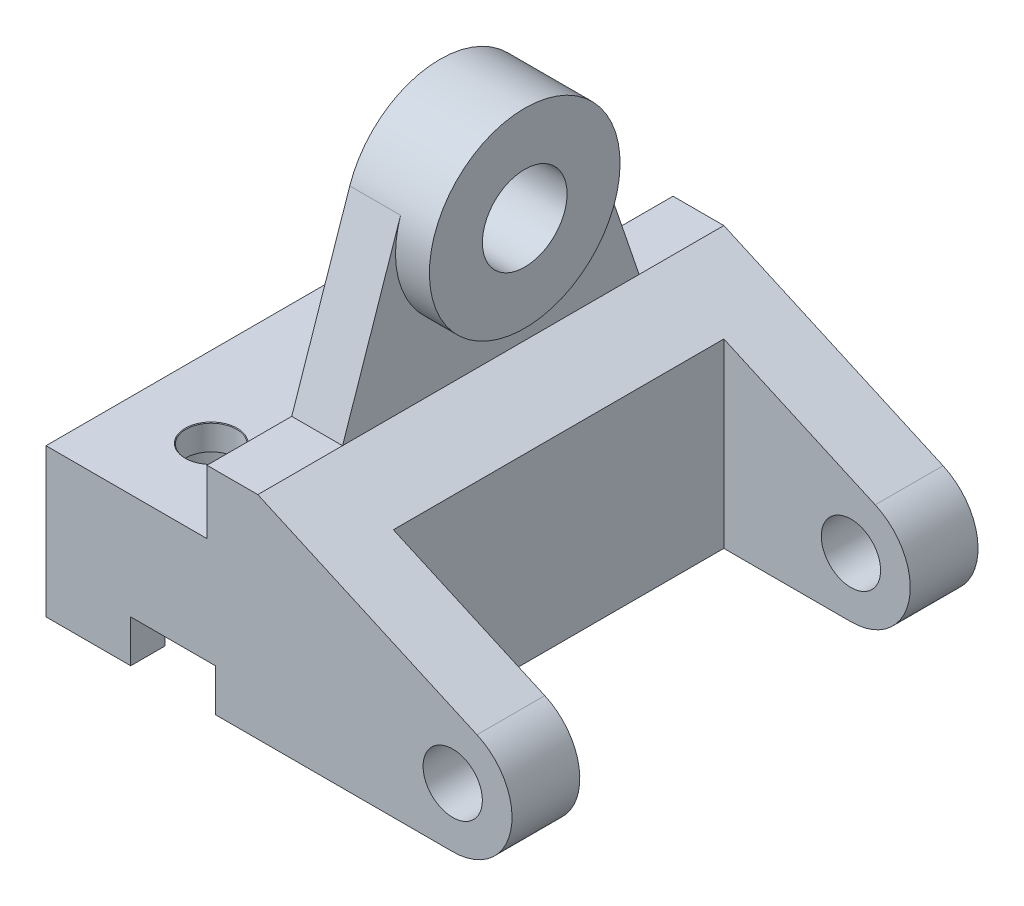
ISO-10303-21;
HEADER;
FILE_DESCRIPTION(('STEP AP214'),'2;1');
FILE_NAME('part.step','',(''),(''),'','','');
FILE_SCHEMA(('AUTOMOTIVE_DESIGN { 1 0 10303 214 1 1 1 1 }'));
ENDSEC;
DATA;
#1=APPLICATION_CONTEXT('core data for automotive mechanical design processes');
#2=APPLICATION_PROTOCOL_DEFINITION('international standard','automotive_design',2000,#1);
#3=PRODUCT_CONTEXT('',#1,'mechanical');
#4=PRODUCT('Part','Part','',(#3));
#5=PRODUCT_RELATED_PRODUCT_CATEGORY('part','',(#4));
#6=PRODUCT_DEFINITION_FORMATION('','',#4);
#7=PRODUCT_DEFINITION_CONTEXT('part definition',#1,'design');
#8=PRODUCT_DEFINITION('design','',#6,#7);
#9=PRODUCT_DEFINITION_SHAPE('','',#8);
#10=(LENGTH_UNIT() NAMED_UNIT(*) SI_UNIT(.MILLI.,.METRE.));
#11=(NAMED_UNIT(*) PLANE_ANGLE_UNIT() SI_UNIT($,.RADIAN.));
#12=(NAMED_UNIT(*) SI_UNIT($,.STERADIAN.) SOLID_ANGLE_UNIT());
#13=UNCERTAINTY_MEASURE_WITH_UNIT(LENGTH_MEASURE(1.E-05),#10,'distance_accuracy_value','');
#14=(GEOMETRIC_REPRESENTATION_CONTEXT(3) GLOBAL_UNCERTAINTY_ASSIGNED_CONTEXT((#13)) GLOBAL_UNIT_ASSIGNED_CONTEXT((#10,
#11,#12)) REPRESENTATION_CONTEXT('',''));
#15=CARTESIAN_POINT('',(0.,0.,0.));
#16=DIRECTION('',(0.,0.,1.));
#17=DIRECTION('',(1.,0.,0.));
#18=AXIS2_PLACEMENT_3D('',#15,#16,#17);
#19=CARTESIAN_POINT('',(-28.,0.,-55.));
#20=DIRECTION('',(-1.,0.,0.));
#21=DIRECTION('',(0.,0.,1.));
#22=AXIS2_PLACEMENT_3D('',#19,#20,#21);
#23=PLANE('',#22);
#24=DIRECTION('',(0.,0.,1.));
#25=VECTOR('',#24,1.);
#26=CARTESIAN_POINT('',(-28.,0.,-55.));
#27=LINE('',#26,#25);
#28=CARTESIAN_POINT('',(-28.,0.,46.9582607431014));
#29=VERTEX_POINT('',#28);
#30=CARTESIAN_POINT('',(-28.,0.,55.));
#31=VERTEX_POINT('',#30);
#32=EDGE_CURVE('E213',#29,#31,#27,.T.);
#33=ORIENTED_EDGE('',*,*,#32,.F.);
#34=DIRECTION('',(0.,1.,0.));
#35=VECTOR('',#34,1.);
#36=CARTESIAN_POINT('',(-28.,35.,46.9582607431014));
#37=LINE('',#36,#35);
#38=CARTESIAN_POINT('',(-28.,10.,46.9582607431014));
#39=VERTEX_POINT('',#38);
#40=EDGE_CURVE('E57',#29,#39,#37,.T.);
#41=ORIENTED_EDGE('',*,*,#40,.T.);
#42=DIRECTION('',(0.,0.,1.));
#43=VECTOR('',#42,1.);
#44=CARTESIAN_POINT('',(-28.,10.,-55.));
#45=LINE('',#44,#43);
#46=CARTESIAN_POINT('',(-28.,10.,55.));
#47=VERTEX_POINT('',#46);
#48=EDGE_CURVE('E222',#39,#47,#45,.T.);
#49=ORIENTED_EDGE('',*,*,#48,.T.);
#50=DIRECTION('',(0.,-1.,0.));
#51=VECTOR('',#50,1.);
#52=CARTESIAN_POINT('',(-28.,0.,55.));
#53=LINE('',#52,#51);
#54=EDGE_CURVE('E220',#47,#31,#53,.T.);
#55=ORIENTED_EDGE('',*,*,#54,.T.);
#56=EDGE_LOOP('',(#33,#41,#49,#55));
#57=FACE_BOUND('',#56,.T.);
#58=ADVANCED_FACE('F41',(#57),#23,.F.);
#59=CARTESIAN_POINT('',(-28.,10.,11.9582607431014));
#60=VERTEX_POINT('',#59);
#61=CARTESIAN_POINT('',(-28.,10.,23.0417392568986));
#62=VERTEX_POINT('',#61);
#63=EDGE_CURVE('E206',#60,#62,#45,.T.);
#64=ORIENTED_EDGE('',*,*,#63,.T.);
#65=DIRECTION('',(0.,1.,0.));
#66=VECTOR('',#65,1.);
#67=CARTESIAN_POINT('',(-28.,35.,23.0417392568986));
#68=LINE('',#67,#66);
#69=CARTESIAN_POINT('',(-28.,0.,23.0417392568986));
#70=VERTEX_POINT('',#69);
#71=EDGE_CURVE('E192',#62,#70,#68,.F.);
#72=ORIENTED_EDGE('',*,*,#71,.T.);
#73=CARTESIAN_POINT('',(-28.,0.,11.9582607431014));
#74=VERTEX_POINT('',#73);
#75=EDGE_CURVE('E207',#74,#70,#27,.T.);
#76=ORIENTED_EDGE('',*,*,#75,.F.);
#77=DIRECTION('',(0.,1.,0.));
#78=VECTOR('',#77,1.);
#79=CARTESIAN_POINT('',(-28.,35.,11.9582607431014));
#80=LINE('',#79,#78);
#81=EDGE_CURVE('E198',#74,#60,#80,.T.);
#82=ORIENTED_EDGE('',*,*,#81,.T.);
#83=EDGE_LOOP('',(#64,#72,#76,#82));
#84=FACE_BOUND('',#83,.T.);
#85=ADVANCED_FACE('F202',(#84),#23,.F.);
#86=CARTESIAN_POINT('',(0.,50.,0.));
#87=DIRECTION('',(0.,1.,0.));
#88=DIRECTION('',(0.,0.,1.));
#89=AXIS2_PLACEMENT_3D('',#86,#87,#88);
#90=PLANE('',#89);
#91=DIRECTION('',(1.,0.,0.));
#92=VECTOR('',#91,1.);
#93=CARTESIAN_POINT('',(-10.,50.,-35.));
#94=LINE('',#93,#92);
#95=CARTESIAN_POINT('',(-10.,50.,-35.));
#96=VERTEX_POINT('',#95);
#97=CARTESIAN_POINT('',(1.99999999999997,50.,-35.));
#98=VERTEX_POINT('',#97);
#99=EDGE_CURVE('E313',#96,#98,#94,.T.);
#100=ORIENTED_EDGE('',*,*,#99,.T.);
#101=DIRECTION('',(0.,0.,-1.));
#102=VECTOR('',#101,1.);
#103=CARTESIAN_POINT('',(1.99999999999997,50.,-39.));
#104=LINE('',#103,#102);
#105=CARTESIAN_POINT('',(1.99999999999997,50.,-55.));
#106=VERTEX_POINT('',#105);
#107=EDGE_CURVE('E343',#98,#106,#104,.T.);
#108=ORIENTED_EDGE('',*,*,#107,.T.);
#109=DIRECTION('',(-1.,0.,0.));
#110=VECTOR('',#109,1.);
#111=CARTESIAN_POINT('',(1.99999999999997,50.,-55.));
#112=LINE('',#111,#110);
#113=CARTESIAN_POINT('',(-10.,50.,-55.));
#114=VERTEX_POINT('',#113);
#115=EDGE_CURVE('E302',#106,#114,#112,.T.);
#116=ORIENTED_EDGE('',*,*,#115,.T.);
#117=DIRECTION('',(0.,0.,1.));
#118=VECTOR('',#117,1.);
#119=CARTESIAN_POINT('',(-10.,50.,-55.));
#120=LINE('',#119,#118);
#121=EDGE_CURVE('E294',#114,#96,#120,.T.);
#122=ORIENTED_EDGE('',*,*,#121,.T.);
#123=EDGE_LOOP('',(#100,#108,#116,#122));
#124=FACE_BOUND('',#123,.T.);
#125=ADVANCED_FACE('F479',(#124),#90,.T.);
#126=CARTESIAN_POINT('',(1.99999999999993,222.670755580085,-55.));
#127=DIRECTION('',(1.,0.,0.));
#128=DIRECTION('',(0.,1.,0.));
#129=AXIS2_PLACEMENT_3D('',#126,#127,#128);
#130=PLANE('',#129);
#131=DIRECTION('',(0.,-0.946664750253945,0.322220189663275));
#132=VECTOR('',#131,1.);
#133=CARTESIAN_POINT('',(1.99999999999997,50.,35.));
#134=LINE('',#133,#132);
#135=CARTESIAN_POINT('',(1.99999999999996,90.2499542674237,21.2999568807138));
#136=VERTEX_POINT('',#135);
#137=CARTESIAN_POINT('',(1.99999999999997,50.,35.));
#138=VERTEX_POINT('',#137);
#139=EDGE_CURVE('E321',#136,#138,#134,.T.);
#140=ORIENTED_EDGE('',*,*,#139,.T.);
#141=DIRECTION('',(0.,0.,1.));
#142=VECTOR('',#141,1.);
#143=CARTESIAN_POINT('',(1.99999999999998,50.,39.));
#144=LINE('',#143,#142);
#145=EDGE_CURVE('E401',#98,#138,#144,.T.);
#146=ORIENTED_EDGE('',*,*,#145,.F.);
#147=DIRECTION('',(0.,0.946664750253945,0.322220189663275));
#148=VECTOR('',#147,1.);
#149=CARTESIAN_POINT('',(1.99999999999996,90.2499542674237,-21.2999568807138));
#150=LINE('',#149,#148);
#151=CARTESIAN_POINT('',(1.99999999999996,90.2499542674237,-21.2999568807138));
#152=VERTEX_POINT('',#151);
#153=EDGE_CURVE('E319',#98,#152,#150,.T.);
#154=ORIENTED_EDGE('',*,*,#153,.T.);
#155=CARTESIAN_POINT('',(1.99999999999996,83.,0.));
#156=DIRECTION('',(1.,0.,0.));
#157=DIRECTION('',(0.,1.,0.));
#158=AXIS2_PLACEMENT_3D('',#155,#156,#157);
#159=CIRCLE('',#158,22.5);
#160=EDGE_CURVE('E335',#136,#152,#159,.T.);
#161=ORIENTED_EDGE('',*,*,#160,.F.);
#162=EDGE_LOOP('',(#140,#146,#154,#161));
#163=FACE_BOUND('',#162,.T.);
#164=ADVANCED_FACE('F439',(#163),#130,.T.);
#165=CARTESIAN_POINT('',(48.,35.,55.));
#166=DIRECTION('',(0.,-1.,0.));
#167=DIRECTION('',(1.,0.,0.));
#168=AXIS2_PLACEMENT_3D('',#165,#166,#167);
#169=PLANE('',#168);
#170=CARTESIAN_POINT('',(-29.,35.,35.));
#171=DIRECTION('',(0.,1.,0.));
#172=DIRECTION('',(0.,0.,1.));
#173=AXIS2_PLACEMENT_3D('',#170,#171,#172);
#174=CIRCLE('',#173,6.145);
#175=CARTESIAN_POINT('',(-29.,35.,41.145));
#176=VERTEX_POINT('',#175);
#177=EDGE_CURVE('E435',#176,#176,#174,.T.);
#178=ORIENTED_EDGE('',*,*,#177,.F.);
#179=EDGE_LOOP('',(#178));
#180=FACE_BOUND('',#179,.T.);
#181=CARTESIAN_POINT('',(-29.,35.,0.));
#182=DIRECTION('',(0.,1.,0.));
#183=DIRECTION('',(0.,0.,1.));
#184=AXIS2_PLACEMENT_3D('',#181,#182,#183);
#185=CIRCLE('',#184,6.145);
#186=CARTESIAN_POINT('',(-29.,35.,6.145));
#187=VERTEX_POINT('',#186);
#188=EDGE_CURVE('E419',#187,#187,#185,.T.);
#189=ORIENTED_EDGE('',*,*,#188,.F.);
#190=EDGE_LOOP('',(#189));
#191=FACE_BOUND('',#190,.T.);
#192=DIRECTION('',(0.,0.,-1.));
#193=VECTOR('',#192,1.);
#194=CARTESIAN_POINT('',(-48.,35.,55.));
#195=LINE('',#194,#193);
#196=CARTESIAN_POINT('',(-48.,35.,55.));
#197=VERTEX_POINT('',#196);
#198=CARTESIAN_POINT('',(-48.,35.,-55.));
#199=VERTEX_POINT('',#198);
#200=EDGE_CURVE('E247',#197,#199,#195,.T.);
#201=ORIENTED_EDGE('',*,*,#200,.F.);
#202=DIRECTION('',(-1.,0.,0.));
#203=VECTOR('',#202,1.);
#204=CARTESIAN_POINT('',(48.,35.,55.));
#205=LINE('',#204,#203);
#206=CARTESIAN_POINT('',(-10.,35.,55.));
#207=VERTEX_POINT('',#206);
#208=EDGE_CURVE('E229',#207,#197,#205,.T.);
#209=ORIENTED_EDGE('',*,*,#208,.F.);
#210=DIRECTION('',(0.,0.,1.));
#211=VECTOR('',#210,1.);
#212=CARTESIAN_POINT('',(-10.,35.,-55.));
#213=LINE('',#212,#211);
#214=CARTESIAN_POINT('',(-10.,35.,-55.));
#215=VERTEX_POINT('',#214);
#216=EDGE_CURVE('E296',#215,#207,#213,.T.);
#217=ORIENTED_EDGE('',*,*,#216,.F.);
#218=DIRECTION('',(-1.,0.,0.));
#219=VECTOR('',#218,1.);
#220=CARTESIAN_POINT('',(48.,35.,-55.));
#221=LINE('',#220,#219);
#222=EDGE_CURVE('E216',#215,#199,#221,.T.);
#223=ORIENTED_EDGE('',*,*,#222,.T.);
#224=EDGE_LOOP('',(#201,#209,#217,#223));
#225=FACE_BOUND('',#224,.T.);
#226=ADVANCED_FACE('F43',(#180,#191,#225),#169,.F.);
#227=CARTESIAN_POINT('',(-48.,0.,55.));
#228=DIRECTION('',(0.,1.,0.));
#229=DIRECTION('',(0.,0.,1.));
#230=AXIS2_PLACEMENT_3D('',#227,#228,#229);
#231=PLANE('',#230);
#232=ORIENTED_EDGE('',*,*,#75,.T.);
#233=CARTESIAN_POINT('',(-29.,0.,35.));
#234=DIRECTION('',(0.,1.,0.));
#235=DIRECTION('',(0.,0.,1.));
#236=AXIS2_PLACEMENT_3D('',#233,#234,#235);
#237=CIRCLE('',#236,12.);
#238=EDGE_CURVE('E47',#70,#29,#237,.T.);
#239=ORIENTED_EDGE('',*,*,#238,.T.);
#240=ORIENTED_EDGE('',*,*,#32,.T.);
#241=DIRECTION('',(1.,0.,0.));
#242=VECTOR('',#241,1.);
#243=CARTESIAN_POINT('',(-48.,0.,55.));
#244=LINE('',#243,#242);
#245=CARTESIAN_POINT('',(-48.,0.,55.));
#246=VERTEX_POINT('',#245);
#247=EDGE_CURVE('E236',#246,#31,#244,.T.);
#248=ORIENTED_EDGE('',*,*,#247,.F.);
#249=DIRECTION('',(0.,0.,-1.));
#250=VECTOR('',#249,1.);
#251=CARTESIAN_POINT('',(-48.,0.,55.));
#252=LINE('',#251,#250);
#253=CARTESIAN_POINT('',(-48.,0.,-55.));
#254=VERTEX_POINT('',#253);
#255=EDGE_CURVE('E237',#246,#254,#252,.T.);
#256=ORIENTED_EDGE('',*,*,#255,.T.);
#257=DIRECTION('',(1.,0.,0.));
#258=VECTOR('',#257,1.);
#259=CARTESIAN_POINT('',(-48.,0.,-55.));
#260=LINE('',#259,#258);
#261=CARTESIAN_POINT('',(-28.,0.,-55.));
#262=VERTEX_POINT('',#261);
#263=EDGE_CURVE('E231',#254,#262,#260,.T.);
#264=ORIENTED_EDGE('',*,*,#263,.T.);
#265=CARTESIAN_POINT('',(-28.,0.,-11.9582607431014));
#266=VERTEX_POINT('',#265);
#267=EDGE_CURVE('E215',#262,#266,#27,.T.);
#268=ORIENTED_EDGE('',*,*,#267,.T.);
#269=CARTESIAN_POINT('',(-29.,0.,0.));
#270=DIRECTION('',(0.,1.,0.));
#271=DIRECTION('',(0.,0.,1.));
#272=AXIS2_PLACEMENT_3D('',#269,#270,#271);
#273=CIRCLE('',#272,12.);
#274=EDGE_CURVE('E63',#266,#74,#273,.T.);
#275=ORIENTED_EDGE('',*,*,#274,.T.);
#276=EDGE_LOOP('',(#232,#239,#240,#248,#256,#264,#268,#275));
#277=FACE_BOUND('',#276,.T.);
#278=ADVANCED_FACE('F214',(#277),#231,.F.);
#279=CARTESIAN_POINT('',(-7.99999999999999,0.,55.));
#280=VERTEX_POINT('',#279);
#281=CARTESIAN_POINT('',(48.,0.,55.));
#282=VERTEX_POINT('',#281);
#283=EDGE_CURVE('E232',#280,#282,#244,.T.);
#284=ORIENTED_EDGE('',*,*,#283,.F.);
#285=DIRECTION('',(0.,0.,1.));
#286=VECTOR('',#285,1.);
#287=CARTESIAN_POINT('',(-7.99999999999999,0.,-55.));
#288=LINE('',#287,#286);
#289=CARTESIAN_POINT('',(-7.99999999999999,0.,-55.));
#290=VERTEX_POINT('',#289);
#291=EDGE_CURVE('E227',#290,#280,#288,.T.);
#292=ORIENTED_EDGE('',*,*,#291,.F.);
#293=CARTESIAN_POINT('',(48.,0.,-55.));
#294=VERTEX_POINT('',#293);
#295=EDGE_CURVE('E243',#290,#294,#260,.T.);
#296=ORIENTED_EDGE('',*,*,#295,.T.);
#297=DIRECTION('',(0.,0.,-1.));
#298=VECTOR('',#297,1.);
#299=CARTESIAN_POINT('',(48.,0.,-39.));
#300=LINE('',#299,#298);
#301=CARTESIAN_POINT('',(48.,0.,-39.));
#302=VERTEX_POINT('',#301);
#303=EDGE_CURVE('E344',#302,#294,#300,.T.);
#304=ORIENTED_EDGE('',*,*,#303,.F.);
#305=DIRECTION('',(-1.,0.,0.));
#306=VECTOR('',#305,1.);
#307=CARTESIAN_POINT('',(-7.99999999999999,0.,-39.));
#308=LINE('',#307,#306);
#309=CARTESIAN_POINT('',(18.,0.,-39.));
#310=VERTEX_POINT('',#309);
#311=EDGE_CURVE('E349',#302,#310,#308,.T.);
#312=ORIENTED_EDGE('',*,*,#311,.T.);
#313=DIRECTION('',(0.,0.,-1.));
#314=VECTOR('',#313,1.);
#315=CARTESIAN_POINT('',(18.,0.,-39.));
#316=LINE('',#315,#314);
#317=CARTESIAN_POINT('',(18.,0.,39.));
#318=VERTEX_POINT('',#317);
#319=EDGE_CURVE('E399',#318,#310,#316,.T.);
#320=ORIENTED_EDGE('',*,*,#319,.F.);
#321=DIRECTION('',(1.,0.,0.));
#322=VECTOR('',#321,1.);
#323=CARTESIAN_POINT('',(-7.99999999999999,0.,39.));
#324=LINE('',#323,#322);
#325=CARTESIAN_POINT('',(48.,0.,39.));
#326=VERTEX_POINT('',#325);
#327=EDGE_CURVE('E372',#318,#326,#324,.T.);
#328=ORIENTED_EDGE('',*,*,#327,.T.);
#329=DIRECTION('',(0.,0.,1.));
#330=VECTOR('',#329,1.);
#331=CARTESIAN_POINT('',(48.,0.,39.));
#332=LINE('',#331,#330);
#333=EDGE_CURVE('E366',#326,#282,#332,.T.);
#334=ORIENTED_EDGE('',*,*,#333,.T.);
#335=EDGE_LOOP('',(#284,#292,#296,#304,#312,#320,#328,#334));
#336=FACE_BOUND('',#335,.T.);
#337=ADVANCED_FACE('F497',(#336),#231,.F.);
#338=CARTESIAN_POINT('',(-48.,35.,55.));
#339=DIRECTION('',(1.,0.,0.));
#340=DIRECTION('',(0.,1.,0.));
#341=AXIS2_PLACEMENT_3D('',#338,#339,#340);
#342=PLANE('',#341);
#343=DIRECTION('',(0.,-1.,0.));
#344=VECTOR('',#343,1.);
#345=CARTESIAN_POINT('',(-48.,35.,-55.));
#346=LINE('',#345,#344);
#347=EDGE_CURVE('E241',#199,#254,#346,.T.);
#348=ORIENTED_EDGE('',*,*,#347,.T.);
#349=ORIENTED_EDGE('',*,*,#255,.F.);
#350=DIRECTION('',(0.,-1.,0.));
#351=VECTOR('',#350,1.);
#352=CARTESIAN_POINT('',(-48.,35.,55.));
#353=LINE('',#352,#351);
#354=EDGE_CURVE('E235',#197,#246,#353,.T.);
#355=ORIENTED_EDGE('',*,*,#354,.F.);
#356=ORIENTED_EDGE('',*,*,#200,.T.);
#357=EDGE_LOOP('',(#348,#349,#355,#356));
#358=FACE_BOUND('',#357,.T.);
#359=ADVANCED_FACE('F448',(#358),#342,.F.);
#360=CARTESIAN_POINT('',(0.,0.,55.));
#361=DIRECTION('',(0.,0.,1.));
#362=DIRECTION('',(1.,0.,0.));
#363=AXIS2_PLACEMENT_3D('',#360,#361,#362);
#364=PLANE('',#363);
#365=CARTESIAN_POINT('',(48.,14.,55.));
#366=DIRECTION('',(0.,0.,1.));
#367=DIRECTION('',(1.,0.,0.));
#368=AXIS2_PLACEMENT_3D('',#365,#366,#367);
#369=CIRCLE('',#368,7.);
#370=CARTESIAN_POINT('',(55.,14.,55.));
#371=VERTEX_POINT('',#370);
#372=EDGE_CURVE('E383',#371,#371,#369,.T.);
#373=ORIENTED_EDGE('',*,*,#372,.F.);
#374=EDGE_LOOP('',(#373));
#375=FACE_BOUND('',#374,.T.);
#376=ORIENTED_EDGE('',*,*,#54,.F.);
#377=DIRECTION('',(-1.,0.,0.));
#378=VECTOR('',#377,1.);
#379=CARTESIAN_POINT('',(-28.,10.,55.));
#380=LINE('',#379,#378);
#381=CARTESIAN_POINT('',(-7.99999999999999,10.,55.));
#382=VERTEX_POINT('',#381);
#383=EDGE_CURVE('E264',#382,#47,#380,.T.);
#384=ORIENTED_EDGE('',*,*,#383,.F.);
#385=DIRECTION('',(0.,1.,0.));
#386=VECTOR('',#385,1.);
#387=CARTESIAN_POINT('',(-7.99999999999999,10.,55.));
#388=LINE('',#387,#386);
#389=EDGE_CURVE('E268',#280,#382,#388,.T.);
#390=ORIENTED_EDGE('',*,*,#389,.F.);
#391=ORIENTED_EDGE('',*,*,#283,.T.);
#392=CARTESIAN_POINT('',(48.,14.,55.));
#393=DIRECTION('',(0.,0.,1.));
#394=DIRECTION('',(1.,0.,0.));
#395=AXIS2_PLACEMENT_3D('',#392,#393,#394);
#396=CIRCLE('',#395,14.);
#397=CARTESIAN_POINT('',(53.7343883081993,26.7717183938101,55.));
#398=VERTEX_POINT('',#397);
#399=EDGE_CURVE('E374',#282,#398,#396,.T.);
#400=ORIENTED_EDGE('',*,*,#399,.T.);
#401=DIRECTION('',(-0.912265599557866,0.409599164871374,0.));
#402=VECTOR('',#401,1.);
#403=CARTESIAN_POINT('',(53.7343883081992,26.7717183938101,55.));
#404=LINE('',#403,#402);
#405=CARTESIAN_POINT('',(1.99999999999997,50.,55.));
#406=VERTEX_POINT('',#405);
#407=EDGE_CURVE('E371',#398,#406,#404,.T.);
#408=ORIENTED_EDGE('',*,*,#407,.T.);
#409=DIRECTION('',(1.,0.,0.));
#410=VECTOR('',#409,1.);
#411=CARTESIAN_POINT('',(-10.,50.,55.));
#412=LINE('',#411,#410);
#413=CARTESIAN_POINT('',(-10.,50.,55.));
#414=VERTEX_POINT('',#413);
#415=EDGE_CURVE('E293',#414,#406,#412,.T.);
#416=ORIENTED_EDGE('',*,*,#415,.F.);
#417=DIRECTION('',(0.,-1.,0.));
#418=VECTOR('',#417,1.);
#419=CARTESIAN_POINT('',(-10.,50.,55.));
#420=LINE('',#419,#418);
#421=EDGE_CURVE('E286',#414,#207,#420,.T.);
#422=ORIENTED_EDGE('',*,*,#421,.T.);
#423=ORIENTED_EDGE('',*,*,#208,.T.);
#424=ORIENTED_EDGE('',*,*,#354,.T.);
#425=ORIENTED_EDGE('',*,*,#247,.T.);
#426=EDGE_LOOP('',(#376,#384,#390,#391,#400,#408,#416,#422,#423,#424,#425));
#427=FACE_BOUND('',#426,.T.);
#428=ADVANCED_FACE('F267',(#375,#427),#364,.T.);
#429=CARTESIAN_POINT('',(0.,0.,-55.));
#430=DIRECTION('',(0.,0.,1.));
#431=DIRECTION('',(1.,0.,0.));
#432=AXIS2_PLACEMENT_3D('',#429,#430,#431);
#433=PLANE('',#432);
#434=CARTESIAN_POINT('',(48.,14.,-55.));
#435=DIRECTION('',(0.,0.,-1.));
#436=DIRECTION('',(-1.,0.,0.));
#437=AXIS2_PLACEMENT_3D('',#434,#435,#436);
#438=CIRCLE('',#437,7.);
#439=CARTESIAN_POINT('',(41.,14.,-55.));
#440=VERTEX_POINT('',#439);
#441=EDGE_CURVE('E391',#440,#440,#438,.T.);
#442=ORIENTED_EDGE('',*,*,#441,.F.);
#443=EDGE_LOOP('',(#442));
#444=FACE_BOUND('',#443,.T.);
#445=ORIENTED_EDGE('',*,*,#222,.F.);
#446=DIRECTION('',(0.,-1.,0.));
#447=VECTOR('',#446,1.);
#448=CARTESIAN_POINT('',(-10.,50.,-55.));
#449=LINE('',#448,#447);
#450=EDGE_CURVE('E278',#114,#215,#449,.T.);
#451=ORIENTED_EDGE('',*,*,#450,.F.);
#452=ORIENTED_EDGE('',*,*,#115,.F.);
#453=DIRECTION('',(0.912265599557866,-0.409599164871373,0.));
#454=VECTOR('',#453,1.);
#455=CARTESIAN_POINT('',(1.99999999999997,50.,-55.));
#456=LINE('',#455,#454);
#457=CARTESIAN_POINT('',(53.7343883081993,26.7717183938101,-55.));
#458=VERTEX_POINT('',#457);
#459=EDGE_CURVE('E358',#106,#458,#456,.T.);
#460=ORIENTED_EDGE('',*,*,#459,.T.);
#461=CARTESIAN_POINT('',(48.,14.,-55.));
#462=DIRECTION('',(0.,0.,-1.));
#463=DIRECTION('',(-1.,0.,0.));
#464=AXIS2_PLACEMENT_3D('',#461,#462,#463);
#465=CIRCLE('',#464,14.);
#466=EDGE_CURVE('E355',#458,#294,#465,.T.);
#467=ORIENTED_EDGE('',*,*,#466,.T.);
#468=ORIENTED_EDGE('',*,*,#295,.F.);
#469=DIRECTION('',(0.,1.,0.));
#470=VECTOR('',#469,1.);
#471=CARTESIAN_POINT('',(-7.99999999999999,10.,-55.));
#472=LINE('',#471,#470);
#473=CARTESIAN_POINT('',(-7.99999999999999,10.,-55.));
#474=VERTEX_POINT('',#473);
#475=EDGE_CURVE('E272',#290,#474,#472,.T.);
#476=ORIENTED_EDGE('',*,*,#475,.T.);
#477=DIRECTION('',(-1.,0.,0.));
#478=VECTOR('',#477,1.);
#479=CARTESIAN_POINT('',(-28.,10.,-55.));
#480=LINE('',#479,#478);
#481=CARTESIAN_POINT('',(-28.,10.,-55.));
#482=VERTEX_POINT('',#481);
#483=EDGE_CURVE('E271',#474,#482,#480,.T.);
#484=ORIENTED_EDGE('',*,*,#483,.T.);
#485=DIRECTION('',(0.,-1.,0.));
#486=VECTOR('',#485,1.);
#487=CARTESIAN_POINT('',(-28.,0.,-55.));
#488=LINE('',#487,#486);
#489=EDGE_CURVE('E230',#482,#262,#488,.T.);
#490=ORIENTED_EDGE('',*,*,#489,.T.);
#491=ORIENTED_EDGE('',*,*,#263,.F.);
#492=ORIENTED_EDGE('',*,*,#347,.F.);
#493=EDGE_LOOP('',(#445,#451,#452,#460,#467,#468,#476,#484,#490,#491,#492));
#494=FACE_BOUND('',#493,.T.);
#495=ADVANCED_FACE('F451',(#444,#494),#433,.F.);
#496=CARTESIAN_POINT('',(-28.,10.,-11.9582607431014));
#497=VERTEX_POINT('',#496);
#498=EDGE_CURVE('E217',#482,#497,#45,.T.);
#499=ORIENTED_EDGE('',*,*,#498,.T.);
#500=DIRECTION('',(0.,1.,0.));
#501=VECTOR('',#500,1.);
#502=CARTESIAN_POINT('',(-28.,35.,-11.9582607431014));
#503=LINE('',#502,#501);
#504=EDGE_CURVE('E252',#497,#266,#503,.F.);
#505=ORIENTED_EDGE('',*,*,#504,.T.);
#506=ORIENTED_EDGE('',*,*,#267,.F.);
#507=ORIENTED_EDGE('',*,*,#489,.F.);
#508=EDGE_LOOP('',(#499,#505,#506,#507));
#509=FACE_BOUND('',#508,.T.);
#510=ADVANCED_FACE('F452',(#509),#23,.F.);
#511=CARTESIAN_POINT('',(-28.,10.,-55.));
#512=DIRECTION('',(0.,1.,0.));
#513=DIRECTION('',(-1.,0.,0.));
#514=AXIS2_PLACEMENT_3D('',#511,#512,#513);
#515=PLANE('',#514);
#516=ORIENTED_EDGE('',*,*,#48,.F.);
#517=CARTESIAN_POINT('',(-29.,10.,35.));
#518=DIRECTION('',(0.,1.,0.));
#519=DIRECTION('',(-1.,0.,0.));
#520=AXIS2_PLACEMENT_3D('',#517,#518,#519);
#521=CIRCLE('',#520,12.);
#522=EDGE_CURVE('E11',#39,#62,#521,.T.);
#523=ORIENTED_EDGE('',*,*,#522,.T.);
#524=ORIENTED_EDGE('',*,*,#63,.F.);
#525=CARTESIAN_POINT('',(-29.,10.,0.));
#526=DIRECTION('',(0.,1.,0.));
#527=DIRECTION('',(-1.,0.,0.));
#528=AXIS2_PLACEMENT_3D('',#525,#526,#527);
#529=CIRCLE('',#528,12.);
#530=EDGE_CURVE('E256',#60,#497,#529,.T.);
#531=ORIENTED_EDGE('',*,*,#530,.T.);
#532=ORIENTED_EDGE('',*,*,#498,.F.);
#533=ORIENTED_EDGE('',*,*,#483,.F.);
#534=DIRECTION('',(0.,0.,1.));
#535=VECTOR('',#534,1.);
#536=CARTESIAN_POINT('',(-7.99999999999999,10.,-55.));
#537=LINE('',#536,#535);
#538=EDGE_CURVE('E224',#474,#382,#537,.T.);
#539=ORIENTED_EDGE('',*,*,#538,.T.);
#540=ORIENTED_EDGE('',*,*,#383,.T.);
#541=EDGE_LOOP('',(#516,#523,#524,#531,#532,#533,#539,#540));
#542=FACE_BOUND('',#541,.T.);
#543=ADVANCED_FACE('F253',(#542),#515,.F.);
#544=CARTESIAN_POINT('',(-7.99999999999999,10.,-55.));
#545=DIRECTION('',(1.,0.,0.));
#546=DIRECTION('',(0.,1.,0.));
#547=AXIS2_PLACEMENT_3D('',#544,#545,#546);
#548=PLANE('',#547);
#549=ORIENTED_EDGE('',*,*,#389,.T.);
#550=ORIENTED_EDGE('',*,*,#538,.F.);
#551=ORIENTED_EDGE('',*,*,#475,.F.);
#552=ORIENTED_EDGE('',*,*,#291,.T.);
#553=EDGE_LOOP('',(#549,#550,#551,#552));
#554=FACE_BOUND('',#553,.T.);
#555=ADVANCED_FACE('F484',(#554),#548,.F.);
#556=CARTESIAN_POINT('',(-10.,50.,-55.));
#557=DIRECTION('',(1.,0.,0.));
#558=DIRECTION('',(0.,1.,0.));
#559=AXIS2_PLACEMENT_3D('',#556,#557,#558);
#560=PLANE('',#559);
#561=ORIENTED_EDGE('',*,*,#421,.F.);
#562=CARTESIAN_POINT('',(-10.,50.,35.));
#563=VERTEX_POINT('',#562);
#564=EDGE_CURVE('E303',#563,#414,#120,.T.);
#565=ORIENTED_EDGE('',*,*,#564,.F.);
#566=DIRECTION('',(0.,-0.946664750253945,0.322220189663275));
#567=VECTOR('',#566,1.);
#568=CARTESIAN_POINT('',(-10.,50.,35.));
#569=LINE('',#568,#567);
#570=CARTESIAN_POINT('',(-10.,90.2499542674237,21.2999568807138));
#571=VERTEX_POINT('',#570);
#572=EDGE_CURVE('E329',#571,#563,#569,.T.);
#573=ORIENTED_EDGE('',*,*,#572,.F.);
#574=CARTESIAN_POINT('',(-10.,83.,0.));
#575=DIRECTION('',(1.,0.,0.));
#576=DIRECTION('',(0.,1.,0.));
#577=AXIS2_PLACEMENT_3D('',#574,#575,#576);
#578=CIRCLE('',#577,22.5);
#579=CARTESIAN_POINT('',(-10.,90.2499542674237,-21.2999568807138));
#580=VERTEX_POINT('',#579);
#581=EDGE_CURVE('E324',#580,#571,#578,.T.);
#582=ORIENTED_EDGE('',*,*,#581,.F.);
#583=DIRECTION('',(0.,0.946664750253945,0.322220189663275));
#584=VECTOR('',#583,1.);
#585=CARTESIAN_POINT('',(-10.,90.2499542674237,-21.2999568807138));
#586=LINE('',#585,#584);
#587=EDGE_CURVE('E311',#96,#580,#586,.T.);
#588=ORIENTED_EDGE('',*,*,#587,.F.);
#589=ORIENTED_EDGE('',*,*,#121,.F.);
#590=ORIENTED_EDGE('',*,*,#450,.T.);
#591=ORIENTED_EDGE('',*,*,#216,.T.);
#592=EDGE_LOOP('',(#561,#565,#573,#582,#588,#589,#590,#591));
#593=FACE_BOUND('',#592,.T.);
#594=CARTESIAN_POINT('',(-10.,83.,0.));
#595=DIRECTION('',(1.,0.,0.));
#596=DIRECTION('',(0.,1.,0.));
#597=AXIS2_PLACEMENT_3D('',#594,#595,#596);
#598=CIRCLE('',#597,10.);
#599=CARTESIAN_POINT('',(-10.,93.,0.));
#600=VERTEX_POINT('',#599);
#601=EDGE_CURVE('E334',#600,#600,#598,.T.);
#602=ORIENTED_EDGE('',*,*,#601,.T.);
#603=EDGE_LOOP('',(#602));
#604=FACE_BOUND('',#603,.T.);
#605=ADVANCED_FACE('F558',(#593,#604),#560,.F.);
#606=DIRECTION('',(0.,0.,-1.));
#607=VECTOR('',#606,1.);
#608=CARTESIAN_POINT('',(1.99999999999998,50.,55.));
#609=LINE('',#608,#607);
#610=EDGE_CURVE('E299',#406,#138,#609,.T.);
#611=ORIENTED_EDGE('',*,*,#610,.T.);
#612=DIRECTION('',(1.,0.,0.));
#613=VECTOR('',#612,1.);
#614=CARTESIAN_POINT('',(-10.,50.,35.));
#615=LINE('',#614,#613);
#616=EDGE_CURVE('E309',#563,#138,#615,.T.);
#617=ORIENTED_EDGE('',*,*,#616,.F.);
#618=ORIENTED_EDGE('',*,*,#564,.T.);
#619=ORIENTED_EDGE('',*,*,#415,.T.);
#620=EDGE_LOOP('',(#611,#617,#618,#619));
#621=FACE_BOUND('',#620,.T.);
#622=ADVANCED_FACE('F513',(#621),#90,.T.);
#623=CARTESIAN_POINT('',(-10.,83.,0.));
#624=DIRECTION('',(1.,0.,0.));
#625=DIRECTION('',(0.,1.,0.));
#626=AXIS2_PLACEMENT_3D('',#623,#624,#625);
#627=CYLINDRICAL_SURFACE('',#626,22.5);
#628=DIRECTION('',(1.,0.,0.));
#629=VECTOR('',#628,1.);
#630=CARTESIAN_POINT('',(-10.,90.2499542674237,21.2999568807138));
#631=LINE('',#630,#629);
#632=EDGE_CURVE('E310',#571,#136,#631,.T.);
#633=ORIENTED_EDGE('',*,*,#632,.T.);
#634=ORIENTED_EDGE('',*,*,#160,.T.);
#635=DIRECTION('',(1.,0.,0.));
#636=VECTOR('',#635,1.);
#637=CARTESIAN_POINT('',(-10.,90.2499542674237,-21.2999568807138));
#638=LINE('',#637,#636);
#639=EDGE_CURVE('E297',#580,#152,#638,.T.);
#640=ORIENTED_EDGE('',*,*,#639,.F.);
#641=ORIENTED_EDGE('',*,*,#581,.T.);
#642=EDGE_LOOP('',(#633,#634,#640,#641));
#643=FACE_BOUND('',#642,.T.);
#644=CARTESIAN_POINT('',(9.99999999999996,83.,0.));
#645=DIRECTION('',(1.,0.,0.));
#646=DIRECTION('',(0.,1.,0.));
#647=AXIS2_PLACEMENT_3D('',#644,#645,#646);
#648=CIRCLE('',#647,22.5);
#649=CARTESIAN_POINT('',(9.99999999999996,105.5,0.));
#650=VERTEX_POINT('',#649);
#651=EDGE_CURVE('E322',#650,#650,#648,.T.);
#652=ORIENTED_EDGE('',*,*,#651,.F.);
#653=EDGE_LOOP('',(#652));
#654=FACE_BOUND('',#653,.T.);
#655=ADVANCED_FACE('F509',(#643,#654),#627,.T.);
#656=CARTESIAN_POINT('',(-10.,90.2499542674237,-21.2999568807138));
#657=DIRECTION('',(0.,0.322220189663275,-0.946664750253944));
#658=DIRECTION('',(0.,0.946664750253945,0.322220189663275));
#659=AXIS2_PLACEMENT_3D('',#656,#657,#658);
#660=PLANE('',#659);
#661=ORIENTED_EDGE('',*,*,#153,.F.);
#662=ORIENTED_EDGE('',*,*,#99,.F.);
#663=ORIENTED_EDGE('',*,*,#587,.T.);
#664=ORIENTED_EDGE('',*,*,#639,.T.);
#665=EDGE_LOOP('',(#661,#662,#663,#664));
#666=FACE_BOUND('',#665,.T.);
#667=ADVANCED_FACE('F511',(#666),#660,.T.);
#668=CARTESIAN_POINT('',(-10.,50.,35.));
#669=DIRECTION('',(0.,0.322220189663275,0.946664750253945));
#670=DIRECTION('',(0.,-0.946664750253945,0.322220189663275));
#671=AXIS2_PLACEMENT_3D('',#668,#669,#670);
#672=PLANE('',#671);
#673=ORIENTED_EDGE('',*,*,#139,.F.);
#674=ORIENTED_EDGE('',*,*,#632,.F.);
#675=ORIENTED_EDGE('',*,*,#572,.T.);
#676=ORIENTED_EDGE('',*,*,#616,.T.);
#677=EDGE_LOOP('',(#673,#674,#675,#676));
#678=FACE_BOUND('',#677,.T.);
#679=ADVANCED_FACE('F530',(#678),#672,.T.);
#680=CARTESIAN_POINT('',(9.99999999999996,83.,0.));
#681=DIRECTION('',(1.,0.,0.));
#682=DIRECTION('',(0.,1.,0.));
#683=AXIS2_PLACEMENT_3D('',#680,#681,#682);
#684=PLANE('',#683);
#685=CARTESIAN_POINT('',(9.99999999999996,83.,0.));
#686=DIRECTION('',(1.,0.,0.));
#687=DIRECTION('',(0.,1.,0.));
#688=AXIS2_PLACEMENT_3D('',#685,#686,#687);
#689=CIRCLE('',#688,10.);
#690=CARTESIAN_POINT('',(9.99999999999996,93.,0.));
#691=VERTEX_POINT('',#690);
#692=EDGE_CURVE('E336',#691,#691,#689,.T.);
#693=ORIENTED_EDGE('',*,*,#692,.F.);
#694=EDGE_LOOP('',(#693));
#695=FACE_BOUND('',#694,.T.);
#696=ORIENTED_EDGE('',*,*,#651,.T.);
#697=EDGE_LOOP('',(#696));
#698=FACE_BOUND('',#697,.T.);
#699=ADVANCED_FACE('F524',(#695,#698),#684,.T.);
#700=CARTESIAN_POINT('',(-10.,83.,0.));
#701=DIRECTION('',(1.,0.,0.));
#702=DIRECTION('',(0.,1.,0.));
#703=AXIS2_PLACEMENT_3D('',#700,#701,#702);
#704=CYLINDRICAL_SURFACE('',#703,10.);
#705=ORIENTED_EDGE('',*,*,#601,.F.);
#706=EDGE_LOOP('',(#705));
#707=FACE_BOUND('',#706,.T.);
#708=ORIENTED_EDGE('',*,*,#692,.T.);
#709=EDGE_LOOP('',(#708));
#710=FACE_BOUND('',#709,.T.);
#711=ADVANCED_FACE('F526',(#707,#710),#704,.F.);
#712=CARTESIAN_POINT('',(48.,14.,-39.));
#713=DIRECTION('',(0.,0.,-1.));
#714=DIRECTION('',(-1.,0.,0.));
#715=AXIS2_PLACEMENT_3D('',#712,#713,#714);
#716=CYLINDRICAL_SURFACE('',#715,14.);
#717=ORIENTED_EDGE('',*,*,#466,.F.);
#718=DIRECTION('',(0.,0.,-1.));
#719=VECTOR('',#718,1.);
#720=CARTESIAN_POINT('',(53.7343883081993,26.7717183938101,-39.));
#721=LINE('',#720,#719);
#722=CARTESIAN_POINT('',(53.7343883081993,26.7717183938101,-39.));
#723=VERTEX_POINT('',#722);
#724=EDGE_CURVE('E347',#723,#458,#721,.T.);
#725=ORIENTED_EDGE('',*,*,#724,.F.);
#726=CARTESIAN_POINT('',(48.,14.,-39.));
#727=DIRECTION('',(0.,0.,-1.));
#728=DIRECTION('',(-1.,0.,0.));
#729=AXIS2_PLACEMENT_3D('',#726,#727,#728);
#730=CIRCLE('',#729,14.);
#731=EDGE_CURVE('E365',#723,#302,#730,.T.);
#732=ORIENTED_EDGE('',*,*,#731,.T.);
#733=ORIENTED_EDGE('',*,*,#303,.T.);
#734=EDGE_LOOP('',(#717,#725,#732,#733));
#735=FACE_BOUND('',#734,.T.);
#736=ADVANCED_FACE('F539',(#735),#716,.T.);
#737=CARTESIAN_POINT('',(1.99999999999997,50.,-39.));
#738=DIRECTION('',(0.409599164871374,0.912265599557866,0.));
#739=DIRECTION('',(-0.912265599557866,0.409599164871374,0.));
#740=AXIS2_PLACEMENT_3D('',#737,#738,#739);
#741=PLANE('',#740);
#742=ORIENTED_EDGE('',*,*,#459,.F.);
#743=ORIENTED_EDGE('',*,*,#107,.F.);
#744=ORIENTED_EDGE('',*,*,#145,.T.);
#745=ORIENTED_EDGE('',*,*,#610,.F.);
#746=ORIENTED_EDGE('',*,*,#407,.F.);
#747=DIRECTION('',(0.,0.,1.));
#748=VECTOR('',#747,1.);
#749=CARTESIAN_POINT('',(53.7343883081993,26.7717183938101,39.));
#750=LINE('',#749,#748);
#751=CARTESIAN_POINT('',(53.7343883081993,26.7717183938101,39.));
#752=VERTEX_POINT('',#751);
#753=EDGE_CURVE('E360',#752,#398,#750,.T.);
#754=ORIENTED_EDGE('',*,*,#753,.F.);
#755=DIRECTION('',(-0.912265599557866,0.409599164871374,0.));
#756=VECTOR('',#755,1.);
#757=CARTESIAN_POINT('',(53.7343883081992,26.7717183938101,39.));
#758=LINE('',#757,#756);
#759=CARTESIAN_POINT('',(18.,42.8161418767537,39.));
#760=VERTEX_POINT('',#759);
#761=EDGE_CURVE('E367',#752,#760,#758,.T.);
#762=ORIENTED_EDGE('',*,*,#761,.T.);
#763=DIRECTION('',(0.,0.,1.));
#764=VECTOR('',#763,1.);
#765=CARTESIAN_POINT('',(18.,42.8161418767537,-55.001));
#766=LINE('',#765,#764);
#767=CARTESIAN_POINT('',(18.,42.8161418767537,-39.));
#768=VERTEX_POINT('',#767);
#769=EDGE_CURVE('E409',#768,#760,#766,.T.);
#770=ORIENTED_EDGE('',*,*,#769,.F.);
#771=DIRECTION('',(0.912265599557866,-0.409599164871373,0.));
#772=VECTOR('',#771,1.);
#773=CARTESIAN_POINT('',(1.99999999999997,50.,-39.));
#774=LINE('',#773,#772);
#775=EDGE_CURVE('E354',#768,#723,#774,.T.);
#776=ORIENTED_EDGE('',*,*,#775,.T.);
#777=ORIENTED_EDGE('',*,*,#724,.T.);
#778=EDGE_LOOP('',(#742,#743,#744,#745,#746,#754,#762,#770,#776,#777));
#779=FACE_BOUND('',#778,.T.);
#780=ADVANCED_FACE('F546',(#779),#741,.T.);
#781=CARTESIAN_POINT('',(48.,14.,-39.));
#782=DIRECTION('',(0.,0.,-1.));
#783=DIRECTION('',(-1.,0.,0.));
#784=AXIS2_PLACEMENT_3D('',#781,#782,#783);
#785=PLANE('',#784);
#786=CARTESIAN_POINT('',(48.,14.,-39.));
#787=DIRECTION('',(0.,0.,-1.));
#788=DIRECTION('',(-1.,0.,0.));
#789=AXIS2_PLACEMENT_3D('',#786,#787,#788);
#790=CIRCLE('',#789,7.);
#791=CARTESIAN_POINT('',(41.,14.,-39.));
#792=VERTEX_POINT('',#791);
#793=EDGE_CURVE('E390',#792,#792,#790,.T.);
#794=ORIENTED_EDGE('',*,*,#793,.T.);
#795=EDGE_LOOP('',(#794));
#796=FACE_BOUND('',#795,.T.);
#797=ORIENTED_EDGE('',*,*,#775,.F.);
#798=DIRECTION('',(0.,1.,0.));
#799=VECTOR('',#798,1.);
#800=CARTESIAN_POINT('',(18.,0.,-39.));
#801=LINE('',#800,#799);
#802=EDGE_CURVE('E393',#310,#768,#801,.T.);
#803=ORIENTED_EDGE('',*,*,#802,.F.);
#804=ORIENTED_EDGE('',*,*,#311,.F.);
#805=ORIENTED_EDGE('',*,*,#731,.F.);
#806=EDGE_LOOP('',(#797,#803,#804,#805));
#807=FACE_BOUND('',#806,.T.);
#808=ADVANCED_FACE('F573',(#796,#807),#785,.F.);
#809=CARTESIAN_POINT('',(48.,14.,39.));
#810=DIRECTION('',(0.,0.,1.));
#811=DIRECTION('',(1.,0.,0.));
#812=AXIS2_PLACEMENT_3D('',#809,#810,#811);
#813=CYLINDRICAL_SURFACE('',#812,14.);
#814=ORIENTED_EDGE('',*,*,#399,.F.);
#815=ORIENTED_EDGE('',*,*,#333,.F.);
#816=CARTESIAN_POINT('',(48.,14.,39.));
#817=DIRECTION('',(0.,0.,1.));
#818=DIRECTION('',(1.,0.,0.));
#819=AXIS2_PLACEMENT_3D('',#816,#817,#818);
#820=CIRCLE('',#819,14.);
#821=EDGE_CURVE('E382',#326,#752,#820,.T.);
#822=ORIENTED_EDGE('',*,*,#821,.T.);
#823=ORIENTED_EDGE('',*,*,#753,.T.);
#824=EDGE_LOOP('',(#814,#815,#822,#823));
#825=FACE_BOUND('',#824,.T.);
#826=ADVANCED_FACE('F569',(#825),#813,.T.);
#827=CARTESIAN_POINT('',(48.,14.,39.));
#828=DIRECTION('',(0.,0.,1.));
#829=DIRECTION('',(1.,0.,0.));
#830=AXIS2_PLACEMENT_3D('',#827,#828,#829);
#831=PLANE('',#830);
#832=CARTESIAN_POINT('',(48.,14.,39.));
#833=DIRECTION('',(0.,0.,1.));
#834=DIRECTION('',(1.,0.,0.));
#835=AXIS2_PLACEMENT_3D('',#832,#833,#834);
#836=CIRCLE('',#835,7.);
#837=CARTESIAN_POINT('',(55.,14.,39.));
#838=VERTEX_POINT('',#837);
#839=EDGE_CURVE('E377',#838,#838,#836,.T.);
#840=ORIENTED_EDGE('',*,*,#839,.T.);
#841=EDGE_LOOP('',(#840));
#842=FACE_BOUND('',#841,.T.);
#843=ORIENTED_EDGE('',*,*,#327,.F.);
#844=DIRECTION('',(0.,1.,0.));
#845=VECTOR('',#844,1.);
#846=CARTESIAN_POINT('',(18.,0.,39.));
#847=LINE('',#846,#845);
#848=EDGE_CURVE('E400',#318,#760,#847,.T.);
#849=ORIENTED_EDGE('',*,*,#848,.T.);
#850=ORIENTED_EDGE('',*,*,#761,.F.);
#851=ORIENTED_EDGE('',*,*,#821,.F.);
#852=EDGE_LOOP('',(#843,#849,#850,#851));
#853=FACE_BOUND('',#852,.T.);
#854=ADVANCED_FACE('F572',(#842,#853),#831,.F.);
#855=CARTESIAN_POINT('',(48.,14.,39.));
#856=DIRECTION('',(0.,0.,1.));
#857=DIRECTION('',(1.,0.,0.));
#858=AXIS2_PLACEMENT_3D('',#855,#856,#857);
#859=CYLINDRICAL_SURFACE('',#858,7.);
#860=ORIENTED_EDGE('',*,*,#839,.F.);
#861=EDGE_LOOP('',(#860));
#862=FACE_BOUND('',#861,.T.);
#863=ORIENTED_EDGE('',*,*,#372,.T.);
#864=EDGE_LOOP('',(#863));
#865=FACE_BOUND('',#864,.T.);
#866=ADVANCED_FACE('F587',(#862,#865),#859,.F.);
#867=CARTESIAN_POINT('',(48.,14.,-39.));
#868=DIRECTION('',(0.,0.,-1.));
#869=DIRECTION('',(-1.,0.,0.));
#870=AXIS2_PLACEMENT_3D('',#867,#868,#869);
#871=CYLINDRICAL_SURFACE('',#870,7.);
#872=ORIENTED_EDGE('',*,*,#793,.F.);
#873=EDGE_LOOP('',(#872));
#874=FACE_BOUND('',#873,.T.);
#875=ORIENTED_EDGE('',*,*,#441,.T.);
#876=EDGE_LOOP('',(#875));
#877=FACE_BOUND('',#876,.T.);
#878=ADVANCED_FACE('F468',(#874,#877),#871,.F.);
#879=CARTESIAN_POINT('',(18.,0.,-39.));
#880=DIRECTION('',(1.,0.,0.));
#881=DIRECTION('',(0.,0.,-1.));
#882=AXIS2_PLACEMENT_3D('',#879,#880,#881);
#883=PLANE('',#882);
#884=ORIENTED_EDGE('',*,*,#769,.T.);
#885=ORIENTED_EDGE('',*,*,#848,.F.);
#886=ORIENTED_EDGE('',*,*,#319,.T.);
#887=ORIENTED_EDGE('',*,*,#802,.T.);
#888=EDGE_LOOP('',(#884,#885,#886,#887));
#889=FACE_BOUND('',#888,.T.);
#890=ADVANCED_FACE('F458',(#889),#883,.T.);
#891=CARTESIAN_POINT('',(-29.,35.,0.));
#892=DIRECTION('',(0.,1.,0.));
#893=DIRECTION('',(0.,0.,1.));
#894=AXIS2_PLACEMENT_3D('',#891,#892,#893);
#895=CYLINDRICAL_SURFACE('',#894,12.);
#896=CARTESIAN_POINT('',(-29.,29.,0.));
#897=DIRECTION('',(0.,1.,0.));
#898=DIRECTION('',(0.,0.,1.));
#899=AXIS2_PLACEMENT_3D('',#896,#897,#898);
#900=CIRCLE('',#899,12.);
#901=CARTESIAN_POINT('',(-29.,29.,12.));
#902=VERTEX_POINT('',#901);
#903=EDGE_CURVE('E411',#902,#902,#900,.T.);
#904=ORIENTED_EDGE('',*,*,#903,.T.);
#905=EDGE_LOOP('',(#904));
#906=FACE_BOUND('',#905,.T.);
#907=ORIENTED_EDGE('',*,*,#274,.F.);
#908=ORIENTED_EDGE('',*,*,#504,.F.);
#909=ORIENTED_EDGE('',*,*,#530,.F.);
#910=ORIENTED_EDGE('',*,*,#81,.F.);
#911=EDGE_LOOP('',(#907,#908,#909,#910));
#912=FACE_BOUND('',#911,.T.);
#913=ADVANCED_FACE('F456',(#906,#912),#895,.F.);
#914=CARTESIAN_POINT('',(-23.,29.,0.));
#915=DIRECTION('',(0.,1.,0.));
#916=DIRECTION('',(0.,0.,1.));
#917=AXIS2_PLACEMENT_3D('',#914,#915,#916);
#918=PLANE('',#917);
#919=ORIENTED_EDGE('',*,*,#903,.F.);
#920=EDGE_LOOP('',(#919));
#921=FACE_BOUND('',#920,.T.);
#922=CARTESIAN_POINT('',(-29.,29.,0.));
#923=DIRECTION('',(0.,1.,0.));
#924=DIRECTION('',(0.,0.,1.));
#925=AXIS2_PLACEMENT_3D('',#922,#923,#924);
#926=CIRCLE('',#925,6.);
#927=CARTESIAN_POINT('',(-29.,29.,6.));
#928=VERTEX_POINT('',#927);
#929=EDGE_CURVE('E413',#928,#928,#926,.T.);
#930=ORIENTED_EDGE('',*,*,#929,.T.);
#931=EDGE_LOOP('',(#930));
#932=FACE_BOUND('',#931,.T.);
#933=ADVANCED_FACE('F459',(#921,#932),#918,.F.);
#934=CARTESIAN_POINT('',(-29.,35.,0.));
#935=DIRECTION('',(0.,1.,0.));
#936=DIRECTION('',(0.,0.,1.));
#937=AXIS2_PLACEMENT_3D('',#934,#935,#936);
#938=CYLINDRICAL_SURFACE('',#937,6.);
#939=ORIENTED_EDGE('',*,*,#929,.F.);
#940=EDGE_LOOP('',(#939));
#941=FACE_BOUND('',#940,.T.);
#942=CARTESIAN_POINT('',(-29.,34.855,0.));
#943=DIRECTION('',(0.,1.,0.));
#944=DIRECTION('',(0.,0.,1.));
#945=AXIS2_PLACEMENT_3D('',#942,#943,#944);
#946=CIRCLE('',#945,6.);
#947=CARTESIAN_POINT('',(-29.,34.855,6.));
#948=VERTEX_POINT('',#947);
#949=EDGE_CURVE('E420',#948,#948,#946,.T.);
#950=ORIENTED_EDGE('',*,*,#949,.T.);
#951=EDGE_LOOP('',(#950));
#952=FACE_BOUND('',#951,.T.);
#953=ADVANCED_FACE('F467',(#941,#952),#938,.F.);
#954=CARTESIAN_POINT('',(-29.,35.,0.));
#955=DIRECTION('',(0.,1.,0.));
#956=DIRECTION('',(0.,0.,1.));
#957=AXIS2_PLACEMENT_3D('',#954,#955,#956);
#958=CONICAL_SURFACE('',#957,6.145,0.785398163397448);
#959=ORIENTED_EDGE('',*,*,#949,.F.);
#960=EDGE_LOOP('',(#959));
#961=FACE_BOUND('',#960,.T.);
#962=ORIENTED_EDGE('',*,*,#188,.T.);
#963=EDGE_LOOP('',(#962));
#964=FACE_BOUND('',#963,.T.);
#965=ADVANCED_FACE('F694',(#961,#964),#958,.F.);
#966=CARTESIAN_POINT('',(-29.,35.,35.));
#967=DIRECTION('',(0.,1.,0.));
#968=DIRECTION('',(0.,0.,1.));
#969=AXIS2_PLACEMENT_3D('',#966,#967,#968);
#970=CYLINDRICAL_SURFACE('',#969,12.);
#971=CARTESIAN_POINT('',(-29.,29.,35.));
#972=DIRECTION('',(0.,1.,0.));
#973=DIRECTION('',(0.,0.,1.));
#974=AXIS2_PLACEMENT_3D('',#971,#972,#973);
#975=CIRCLE('',#974,12.);
#976=CARTESIAN_POINT('',(-29.,29.,47.));
#977=VERTEX_POINT('',#976);
#978=EDGE_CURVE('E209',#977,#977,#975,.T.);
#979=ORIENTED_EDGE('',*,*,#978,.T.);
#980=EDGE_LOOP('',(#979));
#981=FACE_BOUND('',#980,.T.);
#982=ORIENTED_EDGE('',*,*,#238,.F.);
#983=ORIENTED_EDGE('',*,*,#71,.F.);
#984=ORIENTED_EDGE('',*,*,#522,.F.);
#985=ORIENTED_EDGE('',*,*,#40,.F.);
#986=EDGE_LOOP('',(#982,#983,#984,#985));
#987=FACE_BOUND('',#986,.T.);
#988=ADVANCED_FACE('F193',(#981,#987),#970,.F.);
#989=CARTESIAN_POINT('',(-23.,29.,35.));
#990=DIRECTION('',(0.,1.,0.));
#991=DIRECTION('',(0.,0.,1.));
#992=AXIS2_PLACEMENT_3D('',#989,#990,#991);
#993=PLANE('',#992);
#994=ORIENTED_EDGE('',*,*,#978,.F.);
#995=EDGE_LOOP('',(#994));
#996=FACE_BOUND('',#995,.T.);
#997=CARTESIAN_POINT('',(-29.,29.,35.));
#998=DIRECTION('',(0.,1.,0.));
#999=DIRECTION('',(0.,0.,1.));
#1000=AXIS2_PLACEMENT_3D('',#997,#998,#999);
#1001=CIRCLE('',#1000,6.);
#1002=CARTESIAN_POINT('',(-29.,29.,41.));
#1003=VERTEX_POINT('',#1002);
#1004=EDGE_CURVE('E428',#1003,#1003,#1001,.T.);
#1005=ORIENTED_EDGE('',*,*,#1004,.T.);
#1006=EDGE_LOOP('',(#1005));
#1007=FACE_BOUND('',#1006,.T.);
#1008=ADVANCED_FACE('F713',(#996,#1007),#993,.F.);
#1009=CARTESIAN_POINT('',(-29.,35.,35.));
#1010=DIRECTION('',(0.,1.,0.));
#1011=DIRECTION('',(0.,0.,1.));
#1012=AXIS2_PLACEMENT_3D('',#1009,#1010,#1011);
#1013=CYLINDRICAL_SURFACE('',#1012,6.);
#1014=ORIENTED_EDGE('',*,*,#1004,.F.);
#1015=EDGE_LOOP('',(#1014));
#1016=FACE_BOUND('',#1015,.T.);
#1017=CARTESIAN_POINT('',(-29.,34.855,35.));
#1018=DIRECTION('',(0.,1.,0.));
#1019=DIRECTION('',(0.,0.,1.));
#1020=AXIS2_PLACEMENT_3D('',#1017,#1018,#1019);
#1021=CIRCLE('',#1020,6.);
#1022=CARTESIAN_POINT('',(-29.,34.855,41.));
#1023=VERTEX_POINT('',#1022);
#1024=EDGE_CURVE('E429',#1023,#1023,#1021,.T.);
#1025=ORIENTED_EDGE('',*,*,#1024,.T.);
#1026=EDGE_LOOP('',(#1025));
#1027=FACE_BOUND('',#1026,.T.);
#1028=ADVANCED_FACE('F722',(#1016,#1027),#1013,.F.);
#1029=CARTESIAN_POINT('',(-29.,35.,35.));
#1030=DIRECTION('',(0.,1.,0.));
#1031=DIRECTION('',(0.,0.,1.));
#1032=AXIS2_PLACEMENT_3D('',#1029,#1030,#1031);
#1033=CONICAL_SURFACE('',#1032,6.145,0.785398163397448);
#1034=ORIENTED_EDGE('',*,*,#1024,.F.);
#1035=EDGE_LOOP('',(#1034));
#1036=FACE_BOUND('',#1035,.T.);
#1037=ORIENTED_EDGE('',*,*,#177,.T.);
#1038=EDGE_LOOP('',(#1037));
#1039=FACE_BOUND('',#1038,.T.);
#1040=ADVANCED_FACE('F436',(#1036,#1039),#1033,.F.);
#1041=CLOSED_SHELL('',(#58,#85,#125,#164,#226,#278,#337,#359,#428,#495,#510,#543,#555,#605,#622,
#655,#667,#679,#699,#711,#736,#780,#808,#826,#854,#866,#878,#890,#913,#933,#953,#965,#988,#1008,
#1028,#1040));
#1042=MANIFOLD_SOLID_BREP('B2',#1041);
#1043=ADVANCED_BREP_SHAPE_REPRESENTATION('',(#18,#1042),#14);
#1044=SHAPE_DEFINITION_REPRESENTATION(#9,#1043);
ENDSEC;
END-ISO-10303-21;
